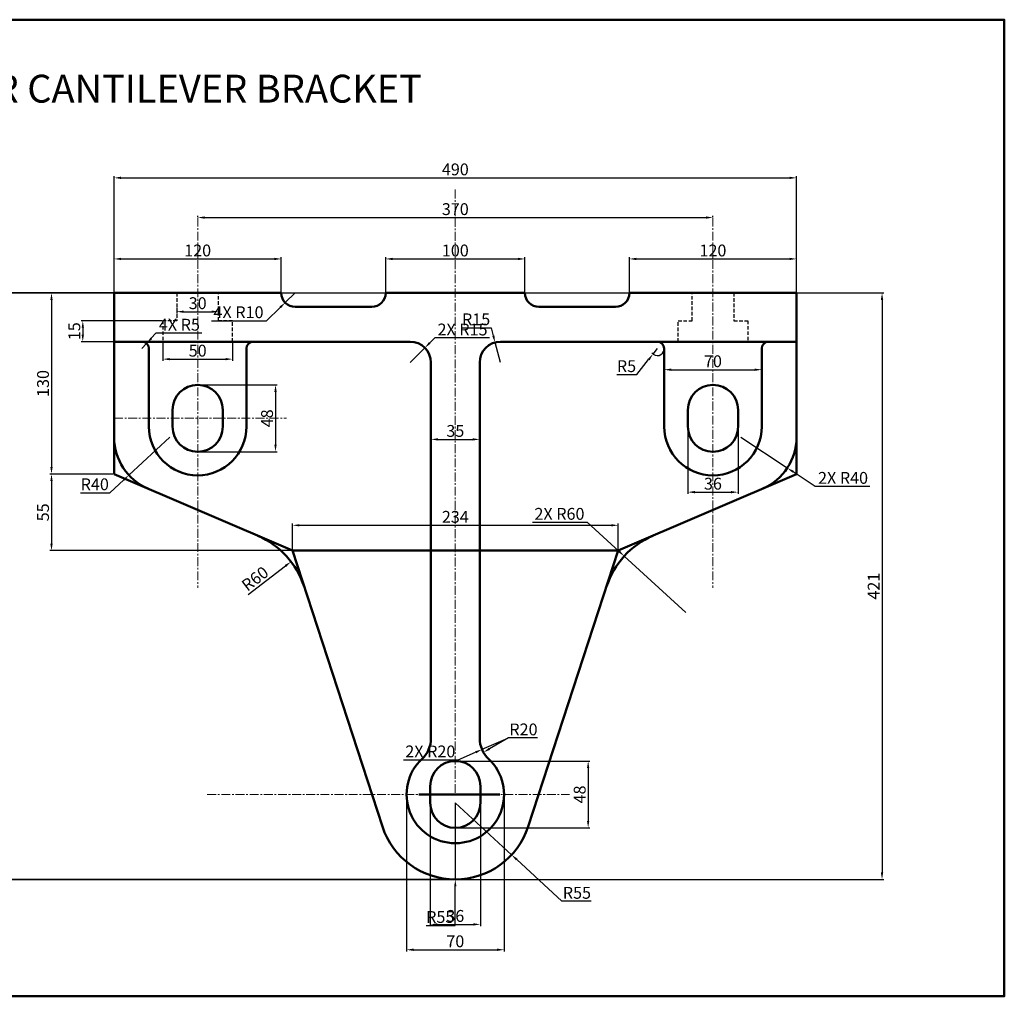
# Model space of a CAD drawing. Units: millimetres. Extents: x -624 to 605, y 670 to 1371.
# Tile 2 of 2: x -102 to 605, y 670 to 1371. Entities that reach past the tile are written whole.
import ezdxf

# ---------------------------------------------------------------- set-up
doc = ezdxf.new("R2010")
doc.units = ezdxf.units.MM
doc.header["$LTSCALE"] = 0.2
doc.linetypes.add('CENTER', pattern=[50.8, 31.75, -6.35, 6.35, -6.35])
doc.linetypes.add('DASHED', pattern=[19.05, 12.7, -6.35])
for name, color, linetype, lineweight in [('M-CNTR', 1, 'CENTER', 18), ('M-DIMS', 2, 'Continuous', 25), ('M-HIDN', 4, 'DASHED', 25), ('M-OUTL', 7, 'Continuous', 50), ('M-TEXT', 7, 'Continuous', 25)]:
    doc.layers.add(name, color=color, linetype=linetype, lineweight=lineweight)
doc.styles.get("Standard").update_dxf_attribs({"font": 'arial.ttf'})
doc.dimstyles.new('ISO-25', dxfattribs={"dimtxt": 8.5, "dimasz": 5, "dimexe": 1.25, "dimexo": 0.625, "dimtad": 1, "dimtoh": 1, "dimtxsty": 'Standard', "dimcen": 2.5, "dimadec": 0, "dimazin": 0, "dimtfac": 1, "dimtmove": 0, "dimatfit": 3, "dimfxl": 1, "dimarcsym": 0})

# ---------------------------------------------------------------- blocks, each defined once
blk = doc.blocks.new('*D22')
at = {"layer": 'Defpoints', "color": 0, "ltscale": 0.2, "transparency": 16777216}
for p in [(85.32, 1198.97), (-34.68, 1174.58), (85.32, 1174.58)]:
    blk.add_point(p, dxfattribs=at)
at = {"layer": 'M-DIMS', "color": 0, "lineweight": -2, "ltscale": 0.2, "transparency": 16777216}
for p, q in [((-34.68, 1175.21), (-34.68, 1200.22)), ((-29.68, 1198.97), (80.32, 1198.97)), ((85.32, 1175.21), (85.32, 1200.22))]:
    blk.add_line(p, q, dxfattribs=at)
at = {"layer": 'M-DIMS', "color": 0, "ltscale": 0.2, "transparency": 16777216}
for points in [[(-29.68, 1199.8), (-29.68, 1198.14), (-34.68, 1198.97)], [(80.32, 1199.8), (80.32, 1198.14), (85.32, 1198.97)]]:
    blk.add_solid(points, dxfattribs=at)
at = {"layer": 'M-DIMS', "color": 0, "ltscale": 0.2, "transparency": 16777216, "insert": (25.32, 1203.94), "char_height": 8.5, "attachment_point": 5}
blk.add_mtext('120', dxfattribs=at)
blk = doc.blocks.new('*D23')
at = {"layer": 'Defpoints', "color": 0, "ltscale": 0.2, "transparency": 16777216}
for p in [(260.32, 1198.97), (160.32, 1174.58), (260.32, 1174.58)]:
    blk.add_point(p, dxfattribs=at)
at = {"layer": 'M-DIMS', "color": 0, "lineweight": -2, "ltscale": 0.2, "transparency": 16777216}
for p, q in [((160.32, 1175.21), (160.32, 1200.22)), ((165.32, 1198.97), (255.32, 1198.97)), ((260.32, 1175.21), (260.32, 1200.22))]:
    blk.add_line(p, q, dxfattribs=at)
at = {"layer": 'M-DIMS', "color": 0, "ltscale": 0.2, "transparency": 16777216}
for points in [[(165.32, 1199.8), (165.32, 1198.14), (160.32, 1198.97)], [(255.32, 1199.8), (255.32, 1198.14), (260.32, 1198.97)]]:
    blk.add_solid(points, dxfattribs=at)
at = {"layer": 'M-DIMS', "color": 0, "ltscale": 0.2, "transparency": 16777216, "insert": (210.32, 1203.94), "char_height": 8.5, "attachment_point": 5}
blk.add_mtext('100', dxfattribs=at)
blk = doc.blocks.new('*D24')
at = {"layer": 'Defpoints', "color": 0, "ltscale": 0.2, "transparency": 16777216}
for p in [(455.32, 1198.97), (335.32, 1174.58), (455.32, 1174.58)]:
    blk.add_point(p, dxfattribs=at)
at = {"layer": 'M-DIMS', "color": 0, "lineweight": -2, "ltscale": 0.2, "transparency": 16777216}
for p, q in [((335.32, 1175.21), (335.32, 1200.22)), ((340.32, 1198.97), (450.32, 1198.97)), ((455.32, 1175.21), (455.32, 1200.22))]:
    blk.add_line(p, q, dxfattribs=at)
at = {"layer": 'M-DIMS', "color": 0, "ltscale": 0.2, "transparency": 16777216}
for points in [[(340.32, 1199.8), (340.32, 1198.14), (335.32, 1198.97)], [(450.32, 1199.8), (450.32, 1198.14), (455.32, 1198.97)]]:
    blk.add_solid(points, dxfattribs=at)
at = {"layer": 'M-DIMS', "color": 0, "ltscale": 0.2, "transparency": 16777216, "insert": (395.32, 1203.94), "char_height": 8.5, "attachment_point": 5}
blk.add_mtext('120', dxfattribs=at)
blk = doc.blocks.new('*D25')
at = {"layer": 'Defpoints', "color": 0, "ltscale": 0.2, "transparency": 16777216}
for p in [(25.32, 1228.67), (395.32, 1228.67), (395.32, 1228.67)]:
    blk.add_point(p, dxfattribs=at)
at = {"layer": 'M-DIMS', "color": 0, "lineweight": -2, "ltscale": 0.2, "transparency": 16777216}
for p, q in [((25.32, 1229.29), (25.32, 1229.92)), ((30.32, 1228.67), (390.32, 1228.67)), ((395.32, 1229.29), (395.32, 1229.92))]:
    blk.add_line(p, q, dxfattribs=at)
at = {"layer": 'M-DIMS', "color": 0, "ltscale": 0.2, "transparency": 16777216}
for points in [[(30.32, 1229.5), (30.32, 1227.83), (25.32, 1228.67)], [(390.32, 1229.5), (390.32, 1227.83), (395.32, 1228.67)]]:
    blk.add_solid(points, dxfattribs=at)
at = {"layer": 'M-DIMS', "color": 0, "ltscale": 0.2, "transparency": 16777216, "insert": (210.32, 1233.63), "char_height": 8.5, "attachment_point": 5}
blk.add_mtext('370', dxfattribs=at)
blk = doc.blocks.new('*D26')
at = {"layer": 'Defpoints', "color": 0, "ltscale": 0.2, "transparency": 16777216}
for p in [(0.32, 1154.58), (-57.18, 1139.58), (0.32, 1139.58)]:
    blk.add_point(p, dxfattribs=at)
at = {"layer": 'M-DIMS', "color": 0, "lineweight": -2, "ltscale": 0.2, "transparency": 16777216}
for p, q in [((-0.3, 1154.58), (-58.43, 1154.58)), ((-57.18, 1149.58), (-57.18, 1144.58)), ((-0.3, 1139.58), (-58.43, 1139.58))]:
    blk.add_line(p, q, dxfattribs=at)
at = {"layer": 'M-DIMS', "color": 0, "ltscale": 0.2, "transparency": 16777216}
for points in [[(-58.01, 1149.58), (-56.35, 1149.58), (-57.18, 1154.58)], [(-58.01, 1144.58), (-56.35, 1144.58), (-57.18, 1139.58)]]:
    blk.add_solid(points, dxfattribs=at)
at = {"layer": 'M-DIMS', "color": 0, "ltscale": 0.2, "transparency": 16777216, "insert": (-62.15, 1147.08), "char_height": 8.5, "attachment_point": 5, "rotation": 90}
blk.add_mtext('15', dxfattribs=at)
blk = doc.blocks.new('*D27')
at = {"layer": 'Defpoints', "color": 0, "ltscale": 0.2, "transparency": 16777216}
for p in [(10.32, 1164.58), (40.32, 1164.58), (40.32, 1161.12)]:
    blk.add_point(p, dxfattribs=at)
at = {"layer": 'M-DIMS', "color": 0, "lineweight": -2, "ltscale": 0.2, "transparency": 16777216}
for p, q in [((10.32, 1163.96), (10.32, 1159.87)), ((15.32, 1161.12), (35.32, 1161.12)), ((40.32, 1163.96), (40.32, 1159.87))]:
    blk.add_line(p, q, dxfattribs=at)
at = {"layer": 'M-DIMS', "color": 0, "ltscale": 0.2, "transparency": 16777216}
for points in [[(15.32, 1161.95), (15.32, 1160.29), (10.32, 1161.12)], [(35.32, 1161.95), (35.32, 1160.29), (40.32, 1161.12)]]:
    blk.add_solid(points, dxfattribs=at)
at = {"layer": 'M-DIMS', "color": 0, "ltscale": 0.2, "transparency": 16777216, "insert": (25.32, 1166.09), "char_height": 8.5, "attachment_point": 5}
blk.add_mtext('30', dxfattribs=at)
blk = doc.blocks.new('*D28')
at = {"layer": 'Defpoints', "color": 0, "ltscale": 0.2, "transparency": 16777216}
for p in [(0.32, 1139.58), (50.32, 1139.58), (50.32, 1127.06)]:
    blk.add_point(p, dxfattribs=at)
at = {"layer": 'M-DIMS', "color": 0, "lineweight": -2, "ltscale": 0.2, "transparency": 16777216}
for p, q in [((0.32, 1138.96), (0.32, 1125.81)), ((50.32, 1138.96), (50.32, 1125.81)), ((5.32, 1127.06), (45.32, 1127.06))]:
    blk.add_line(p, q, dxfattribs=at)
at = {"layer": 'M-DIMS', "color": 0, "ltscale": 0.2, "transparency": 16777216}
for points in [[(5.32, 1127.89), (5.32, 1126.23), (0.32, 1127.06)], [(45.32, 1127.89), (45.32, 1126.23), (50.32, 1127.06)]]:
    blk.add_solid(points, dxfattribs=at)
at = {"layer": 'M-DIMS', "color": 0, "ltscale": 0.2, "transparency": 16777216, "insert": (25.32, 1132.03), "char_height": 8.5, "attachment_point": 5}
blk.add_mtext('50', dxfattribs=at)
blk = doc.blocks.new('*D29')
at = {"layer": 'Defpoints', "color": 0, "ltscale": 0.2, "transparency": 16777216}
for p in [(-34.68, 1174.58), (-79.66, 1044.58), (-34.68, 1044.58)]:
    blk.add_point(p, dxfattribs=at)
at = {"layer": 'M-DIMS', "color": 0, "lineweight": -2, "ltscale": 0.2, "transparency": 16777216}
for p, q in [((-35.3, 1174.58), (-80.91, 1174.58)), ((-79.66, 1169.58), (-79.66, 1049.58)), ((-35.3, 1044.58), (-80.91, 1044.58))]:
    blk.add_line(p, q, dxfattribs=at)
at = {"layer": 'M-DIMS', "color": 0, "ltscale": 0.2, "transparency": 16777216}
for points in [[(-80.49, 1169.58), (-78.83, 1169.58), (-79.66, 1174.58)], [(-80.49, 1049.58), (-78.83, 1049.58), (-79.66, 1044.58)]]:
    blk.add_solid(points, dxfattribs=at)
at = {"layer": 'M-DIMS', "color": 0, "ltscale": 0.2, "transparency": 16777216, "insert": (-84.63, 1109.58), "char_height": 8.5, "attachment_point": 5, "rotation": 90}
blk.add_mtext('130', dxfattribs=at)
blk = doc.blocks.new('*D30')
at = {"layer": 'Defpoints', "color": 0, "ltscale": 0.2, "transparency": 16777216}
for p in [(-34.68, 1044.58), (-79.66, 989.58), (93.32, 989.58)]:
    blk.add_point(p, dxfattribs=at)
at = {"layer": 'M-DIMS', "color": 0, "lineweight": -2, "ltscale": 0.2, "transparency": 16777216}
for p, q in [((-35.3, 1044.58), (-80.91, 1044.58)), ((-79.66, 1039.58), (-79.66, 994.58)), ((92.7, 989.58), (-80.91, 989.58))]:
    blk.add_line(p, q, dxfattribs=at)
at = {"layer": 'M-DIMS', "color": 0, "ltscale": 0.2, "transparency": 16777216}
for points in [[(-80.49, 1039.58), (-78.83, 1039.58), (-79.66, 1044.58)], [(-80.49, 994.58), (-78.83, 994.58), (-79.66, 989.58)]]:
    blk.add_solid(points, dxfattribs=at)
at = {"layer": 'M-DIMS', "color": 0, "ltscale": 0.2, "transparency": 16777216, "insert": (-84.61, 1017.08), "char_height": 8.5, "attachment_point": 5, "rotation": 90}
blk.add_mtext('55', dxfattribs=at)
blk = doc.blocks.new('*D31')
at = {"layer": 'Defpoints', "color": 0, "ltscale": 0.2, "transparency": 16777216}
for p in [(327.32, 1007.77), (93.32, 989.58), (327.32, 989.58)]:
    blk.add_point(p, dxfattribs=at)
at = {"layer": 'M-DIMS', "color": 0, "lineweight": -2, "ltscale": 0.2, "transparency": 16777216}
for p, q in [((93.32, 990.21), (93.32, 1009.02)), ((98.32, 1007.77), (322.32, 1007.77)), ((327.32, 990.21), (327.32, 1009.02))]:
    blk.add_line(p, q, dxfattribs=at)
at = {"layer": 'M-DIMS', "color": 0, "ltscale": 0.2, "transparency": 16777216}
for points in [[(98.32, 1008.61), (98.32, 1006.94), (93.32, 1007.77)], [(322.32, 1008.61), (322.32, 1006.94), (327.32, 1007.77)]]:
    blk.add_solid(points, dxfattribs=at)
at = {"layer": 'M-DIMS', "color": 0, "ltscale": 0.2, "transparency": 16777216, "insert": (210.32, 1012.74), "char_height": 8.5, "attachment_point": 5}
blk.add_mtext('234', dxfattribs=at)
blk = doc.blocks.new('*D32')
at = {"layer": 'Defpoints', "color": 0, "ltscale": 0.2, "transparency": 16777216}
for p in [(192.82, 1076.92), (227.82, 1076.92), (227.82, 1069.44)]:
    blk.add_point(p, dxfattribs=at)
at = {"layer": 'M-DIMS', "color": 0, "lineweight": -2, "ltscale": 0.2, "transparency": 16777216}
for p, q in [((192.82, 1076.29), (192.82, 1068.19)), ((227.82, 1076.29), (227.82, 1068.19)), ((197.82, 1069.44), (222.82, 1069.44))]:
    blk.add_line(p, q, dxfattribs=at)
at = {"layer": 'M-DIMS', "color": 0, "ltscale": 0.2, "transparency": 16777216}
for points in [[(197.82, 1070.28), (197.82, 1068.61), (192.82, 1069.44)], [(222.82, 1070.28), (222.82, 1068.61), (227.82, 1069.44)]]:
    blk.add_solid(points, dxfattribs=at)
at = {"layer": 'M-DIMS', "color": 0, "ltscale": 0.2, "transparency": 16777216, "insert": (210.32, 1074.41), "char_height": 8.5, "attachment_point": 5}
blk.add_mtext('35', dxfattribs=at)
blk = doc.blocks.new('*D33')
at = {"layer": 'Defpoints', "color": 0, "ltscale": 0.2, "transparency": 16777216}
for p in [(192.32, 814.58), (228.32, 814.58), (228.32, 721.31)]:
    blk.add_point(p, dxfattribs=at)
at = {"layer": 'M-DIMS', "color": 0, "lineweight": -2, "ltscale": 0.2, "transparency": 16777216}
for p, q in [((192.32, 813.96), (192.32, 720.06)), ((228.32, 813.96), (228.32, 720.06)), ((197.32, 721.31), (223.32, 721.31))]:
    blk.add_line(p, q, dxfattribs=at)
at = {"layer": 'M-DIMS', "color": 0, "ltscale": 0.2, "transparency": 16777216}
for points in [[(197.32, 722.15), (197.32, 720.48), (192.32, 721.31)], [(223.32, 722.15), (223.32, 720.48), (228.32, 721.31)]]:
    blk.add_solid(points, dxfattribs=at)
at = {"layer": 'M-DIMS', "color": 0, "ltscale": 0.2, "transparency": 16777216, "insert": (210.32, 726.28), "char_height": 8.5, "attachment_point": 5}
blk.add_mtext('36', dxfattribs=at)
blk = doc.blocks.new('*D34')
at = {"layer": 'Defpoints', "color": 0, "ltscale": 0.2, "transparency": 16777216}
for p in [(175.32, 814.58), (245.32, 814.58), (245.32, 703.11)]:
    blk.add_point(p, dxfattribs=at)
at = {"layer": 'M-DIMS', "color": 0, "lineweight": -2, "ltscale": 0.2, "transparency": 16777216}
for p, q in [((175.32, 813.96), (175.32, 701.86)), ((245.32, 813.96), (245.32, 701.86)), ((180.32, 703.11), (240.32, 703.11))]:
    blk.add_line(p, q, dxfattribs=at)
at = {"layer": 'M-DIMS', "color": 0, "ltscale": 0.2, "transparency": 16777216}
for points in [[(180.32, 703.94), (180.32, 702.27), (175.32, 703.11)], [(240.32, 703.94), (240.32, 702.27), (245.32, 703.11)]]:
    blk.add_solid(points, dxfattribs=at)
at = {"layer": 'M-DIMS', "color": 0, "ltscale": 0.2, "transparency": 16777216, "insert": (210.32, 708.07), "char_height": 8.5, "attachment_point": 5}
blk.add_mtext('70', dxfattribs=at)
blk = doc.blocks.new('*D35')
at = {"layer": 'Defpoints', "color": 0, "ltscale": 0.2, "transparency": 16777216}
for p in [(210.32, 838.58), (210.32, 790.58), (305.7, 790.58)]:
    blk.add_point(p, dxfattribs=at)
at = {"layer": 'M-DIMS', "color": 0, "lineweight": -2, "ltscale": 0.2, "transparency": 16777216}
for p, q in [((210.95, 838.58), (306.95, 838.58)), ((305.7, 833.58), (305.7, 795.58)), ((210.95, 790.58), (306.95, 790.58))]:
    blk.add_line(p, q, dxfattribs=at)
at = {"layer": 'M-DIMS', "color": 0, "ltscale": 0.2, "transparency": 16777216}
for points in [[(304.87, 833.58), (306.53, 833.58), (305.7, 838.58)], [(304.87, 795.58), (306.53, 795.58), (305.7, 790.58)]]:
    blk.add_solid(points, dxfattribs=at)
at = {"layer": 'M-DIMS', "color": 0, "ltscale": 0.2, "transparency": 16777216, "insert": (300.74, 814.58), "char_height": 8.5, "attachment_point": 5, "rotation": 90}
blk.add_mtext('48', dxfattribs=at)
blk = doc.blocks.new('*D36')
at = {"layer": 'Defpoints', "color": 0, "ltscale": 0.2, "transparency": 16777216}
for p in [(247.82, 854.81), (230.5, 844.81)]:
    blk.add_point(p, dxfattribs=at)
at = {"layer": 'M-DIMS', "color": 0, "lineweight": -2, "ltscale": 0.2, "transparency": 16777216}
for p, q in [((248.48, 855.2), (234.83, 847.31)), ((269.39, 855.2), (248.48, 855.2))]:
    blk.add_line(p, q, dxfattribs=at)
at = {"layer": 'M-DIMS', "color": 0, "ltscale": 0.2, "transparency": 16777216}
blk.add_solid([(234.41, 848.04), (235.25, 846.59), (230.5, 844.81)], dxfattribs=at)
at = {"layer": 'M-DIMS', "color": 0, "ltscale": 0.2, "transparency": 16777216, "insert": (259.25, 860.16), "char_height": 8.5, "attachment_point": 5}
blk.add_mtext('R20', dxfattribs=at)
blk = doc.blocks.new('*D37')
at = {"layer": 'Defpoints', "color": 0, "ltscale": 0.2, "transparency": 16777216}
for p in [(210.32, 808.58), (250.72, 771.26)]:
    blk.add_point(p, dxfattribs=at)
at = {"layer": 'M-DIMS', "color": 0, "lineweight": -2, "ltscale": 0.2, "transparency": 16777216}
for p, q in [((210.32, 808.58), (250.72, 771.26)), ((286.82, 737.92), (254.4, 767.87)), ((307.82, 737.92), (286.82, 737.92))]:
    blk.add_line(p, q, dxfattribs=at)
at = {"layer": 'M-DIMS', "color": 0, "ltscale": 0.2, "transparency": 16777216}
blk.add_solid([(254.96, 768.48), (253.83, 767.26), (250.72, 771.26)], dxfattribs=at)
at = {"layer": 'M-DIMS', "color": 0, "ltscale": 0.2, "transparency": 16777216, "insert": (297.63, 742.87), "char_height": 8.5, "attachment_point": 5}
blk.add_mtext('R55', dxfattribs=at)
blk = doc.blocks.new('*D38')
at = {"layer": 'Defpoints', "color": 0, "ltscale": 0.2, "transparency": 16777216}
for p in [(92.35, 981.64), (44.71, 945.16)]:
    blk.add_point(p, dxfattribs=at)
at = {"layer": 'M-DIMS', "color": 0, "lineweight": -2, "ltscale": 0.2, "transparency": 16777216}
blk.add_line((61.62, 958.11), (88.38, 978.6), dxfattribs=at)
at = {"layer": 'M-DIMS', "color": 0, "ltscale": 0.2, "transparency": 16777216}
blk.add_solid([(87.87, 979.26), (88.89, 977.94), (92.35, 981.64)], dxfattribs=at)
at = {"layer": 'M-DIMS', "color": 0, "ltscale": 0.2, "transparency": 16777216, "insert": (67.15, 968.6), "char_height": 8.5, "attachment_point": 5, "rotation": 37.44326}
blk.add_mtext('R60', dxfattribs=at)
blk = doc.blocks.new('*D39')
at = {"layer": 'Defpoints', "color": 0, "ltscale": 0.2, "transparency": 16777216}
for p in [(5.32, 1070.93), (-24.08, 1043.81)]:
    blk.add_point(p, dxfattribs=at)
at = {"layer": 'M-DIMS', "color": 0, "lineweight": -2, "ltscale": 0.2, "transparency": 16777216}
for p, q in [((5.32, 1070.93), (-24.08, 1043.81)), ((-37.81, 1031.14), (-27.76, 1040.42)), ((-58.72, 1031.14), (-37.81, 1031.14))]:
    blk.add_line(p, q, dxfattribs=at)
at = {"layer": 'M-DIMS', "color": 0, "ltscale": 0.2, "transparency": 16777216}
blk.add_solid([(-28.32, 1041.03), (-27.19, 1039.81), (-24.08, 1043.81)], dxfattribs=at)
at = {"layer": 'M-DIMS', "color": 0, "ltscale": 0.2, "transparency": 16777216, "insert": (-48.58, 1036.11), "char_height": 8.5, "attachment_point": 5}
blk.add_mtext('R40', dxfattribs=at)
blk = doc.blocks.new('*D40')
at = {"layer": 'Defpoints', "color": 0, "ltscale": 0.2, "transparency": 16777216}
for p in [(25.32, 1108.58), (25.32, 1060.58), (81.21, 1060.58)]:
    blk.add_point(p, dxfattribs=at)
at = {"layer": 'M-DIMS', "color": 0, "lineweight": -2, "ltscale": 0.2, "transparency": 16777216}
for p, q in [((25.95, 1108.58), (82.46, 1108.58)), ((81.21, 1103.58), (81.21, 1065.58)), ((25.95, 1060.58), (82.46, 1060.58))]:
    blk.add_line(p, q, dxfattribs=at)
at = {"layer": 'M-DIMS', "color": 0, "ltscale": 0.2, "transparency": 16777216}
for points in [[(80.37, 1103.58), (82.04, 1103.58), (81.21, 1108.58)], [(80.37, 1065.58), (82.04, 1065.58), (81.21, 1060.58)]]:
    blk.add_solid(points, dxfattribs=at)
at = {"layer": 'M-DIMS', "color": 0, "ltscale": 0.2, "transparency": 16777216, "insert": (76.24, 1084.58), "char_height": 8.5, "attachment_point": 5, "rotation": 90}
blk.add_mtext('48', dxfattribs=at)
blk = doc.blocks.new('*D41')
at = {"layer": 'Defpoints', "color": 0, "ltscale": 0.2, "transparency": 16777216}
for p in [(455.32, 1257.18), (-34.68, 1174.58), (455.32, 1174.58)]:
    blk.add_point(p, dxfattribs=at)
at = {"layer": 'M-DIMS', "color": 0, "lineweight": -2, "ltscale": 0.2, "transparency": 16777216}
for p, q in [((-34.68, 1175.21), (-34.68, 1258.43)), ((-29.68, 1257.18), (450.32, 1257.18)), ((455.32, 1175.21), (455.32, 1258.43))]:
    blk.add_line(p, q, dxfattribs=at)
at = {"layer": 'M-DIMS', "color": 0, "ltscale": 0.2, "transparency": 16777216}
for points in [[(-29.68, 1258.02), (-29.68, 1256.35), (-34.68, 1257.18)], [(450.32, 1258.02), (450.32, 1256.35), (455.32, 1257.18)]]:
    blk.add_solid(points, dxfattribs=at)
at = {"layer": 'M-DIMS', "color": 0, "ltscale": 0.2, "transparency": 16777216, "insert": (210.32, 1262.15), "char_height": 8.5, "attachment_point": 5}
blk.add_mtext('490', dxfattribs=at)
blk = doc.blocks.new('*D42')
at = {"layer": 'Defpoints', "color": 0, "ltscale": 0.2, "transparency": 16777216}
for p in [(360.32, 1118.8), (430.32, 1119.47), (430.32, 1118.8)]:
    blk.add_point(p, dxfattribs=at)
at = {"layer": 'M-DIMS', "color": 0, "lineweight": -2, "ltscale": 0.2, "transparency": 16777216}
for p, q in [((360.32, 1119.42), (360.32, 1120.72)), ((365.32, 1119.47), (425.32, 1119.47)), ((430.32, 1119.42), (430.32, 1120.72))]:
    blk.add_line(p, q, dxfattribs=at)
at = {"layer": 'M-DIMS', "color": 0, "ltscale": 0.2, "transparency": 16777216}
for points in [[(365.32, 1120.3), (365.32, 1118.64), (360.32, 1119.47)], [(425.32, 1120.3), (425.32, 1118.64), (430.32, 1119.47)]]:
    blk.add_solid(points, dxfattribs=at)
at = {"layer": 'M-DIMS', "color": 0, "ltscale": 0.2, "transparency": 16777216, "insert": (395.32, 1124.43), "char_height": 8.5, "attachment_point": 5}
blk.add_mtext('70', dxfattribs=at)
blk = doc.blocks.new('*D43')
at = {"layer": 'Defpoints', "color": 0, "ltscale": 0.2, "transparency": 16777216}
for p in [(377.32, 1084.58), (413.32, 1084.58), (413.32, 1031.58)]:
    blk.add_point(p, dxfattribs=at)
at = {"layer": 'M-DIMS', "color": 0, "lineweight": -2, "ltscale": 0.2, "transparency": 16777216}
for p, q in [((377.32, 1083.96), (377.32, 1030.33)), ((413.32, 1083.96), (413.32, 1030.33)), ((382.32, 1031.58), (408.32, 1031.58))]:
    blk.add_line(p, q, dxfattribs=at)
at = {"layer": 'M-DIMS', "color": 0, "ltscale": 0.2, "transparency": 16777216}
for points in [[(382.32, 1032.41), (382.32, 1030.75), (377.32, 1031.58)], [(408.32, 1032.41), (408.32, 1030.75), (413.32, 1031.58)]]:
    blk.add_solid(points, dxfattribs=at)
at = {"layer": 'M-DIMS', "color": 0, "ltscale": 0.2, "transparency": 16777216, "insert": (395.32, 1036.55), "char_height": 8.5, "attachment_point": 5}
blk.add_mtext('36', dxfattribs=at)
blk = doc.blocks.new('*D44')
at = {"layer": 'Defpoints', "color": 0, "ltscale": 0.2, "transparency": 16777216}
for p in [(355.32, 1134.58), (352.24, 1130.64)]:
    blk.add_point(p, dxfattribs=at)
at = {"layer": 'M-DIMS', "color": 0, "lineweight": -2, "ltscale": 0.2, "transparency": 16777216}
for p, q in [((355.32, 1134.58), (352.24, 1130.64)), ((340.74, 1115.97), (349.15, 1126.71)), ((326.34, 1115.97), (340.74, 1115.97))]:
    blk.add_line(p, q, dxfattribs=at)
blk.add_arc((355.32, 1134.58), 5, 217.60221, 352.83803, dxfattribs=at)
at = {"layer": 'M-DIMS', "color": 0, "ltscale": 0.2, "transparency": 16777216}
blk.add_solid([(348.5, 1127.22), (349.81, 1126.19), (352.24, 1130.64)], dxfattribs=at)
at = {"layer": 'M-DIMS', "color": 0, "ltscale": 0.2, "transparency": 16777216, "insert": (333.23, 1120.91), "char_height": 8.5, "attachment_point": 5}
blk.add_mtext('R5', dxfattribs=at)
blk = doc.blocks.new('*D45')
at = {"layer": 'Defpoints', "color": 0, "ltscale": 0.2, "transparency": 16777216}
for p in [(238.89, 1139.06), (242.82, 1124.58)]:
    blk.add_point(p, dxfattribs=at)
at = {"layer": 'M-DIMS', "color": 0, "lineweight": -2, "ltscale": 0.2, "transparency": 16777216}
for p, q in [((215.05, 1149.54), (236.05, 1149.54)), ((236.05, 1149.54), (237.58, 1143.88)), ((242.82, 1124.58), (238.89, 1139.06))]:
    blk.add_line(p, q, dxfattribs=at)
at = {"layer": 'M-DIMS', "color": 0, "ltscale": 0.2, "transparency": 16777216}
blk.add_solid([(238.39, 1144.1), (236.78, 1143.66), (238.89, 1139.06)], dxfattribs=at)
at = {"layer": 'M-DIMS', "color": 0, "ltscale": 0.2, "transparency": 16777216, "insert": (225.24, 1154.51), "char_height": 8.5, "attachment_point": 5}
blk.add_mtext('R15', dxfattribs=at)
blk = doc.blocks.new('*D47')
at = {"layer": 'Defpoints', "color": 0, "ltscale": 0.2, "transparency": 16777216}
for p in [(-548.12, 1174.58), (-188.12, 753.58), (516.74, 753.58)]:
    blk.add_point(p, dxfattribs=at)
at = {"layer": 'M-DIMS', "color": 0, "lineweight": -2, "ltscale": 0.2, "transparency": 16777216}
for p, q in [((-547.5, 1174.58), (517.99, 1174.58)), ((516.74, 1169.58), (516.74, 758.58)), ((-187.5, 753.58), (517.99, 753.58))]:
    blk.add_line(p, q, dxfattribs=at)
at = {"layer": 'M-DIMS', "color": 0, "ltscale": 0.2, "transparency": 16777216}
for points in [[(515.9, 1169.58), (517.57, 1169.58), (516.74, 1174.58)], [(515.9, 758.58), (517.57, 758.58), (516.74, 753.58)]]:
    blk.add_solid(points, dxfattribs=at)
at = {"layer": 'M-DIMS', "color": 0, "ltscale": 0.2, "transparency": 16777216, "insert": (511.84, 964.08), "char_height": 8.5, "attachment_point": 5, "rotation": 90}
blk.add_mtext('421', dxfattribs=at)
blk = doc.blocks.new('*D48')
at = {"layer": 'Defpoints', "color": 0, "ltscale": 0.2, "transparency": 16777216}
for p in [(-34.68, 1174.58), (-609.54, 753.58), (210.32, 753.58)]:
    blk.add_point(p, dxfattribs=at)
at = {"layer": 'M-DIMS', "color": 0, "lineweight": -2, "ltscale": 0.2, "transparency": 16777216}
for p, q in [((-35.3, 1174.58), (-610.79, 1174.58)), ((-609.54, 1169.58), (-609.54, 758.58)), ((209.7, 753.58), (-610.79, 753.58))]:
    blk.add_line(p, q, dxfattribs=at)
at = {"layer": 'M-DIMS', "color": 0, "ltscale": 0.2, "transparency": 16777216}
for points in [[(-610.37, 1169.58), (-608.71, 1169.58), (-609.54, 1174.58)], [(-610.37, 758.58), (-608.71, 758.58), (-609.54, 753.58)]]:
    blk.add_solid(points, dxfattribs=at)
at = {"layer": 'M-DIMS', "color": 0, "ltscale": 0.2, "transparency": 16777216, "insert": (-614.43, 964.08), "char_height": 8.5, "attachment_point": 5, "rotation": 90}
blk.add_mtext('421', dxfattribs=at)
blk = doc.blocks.new('*D54')
at = {"layer": 'Defpoints', "color": 0, "ltscale": 0.2, "transparency": 16777216}
for p in [(188.43, 1135.19), (177.82, 1124.58)]:
    blk.add_point(p, dxfattribs=at)
at = {"layer": 'M-DIMS', "color": 0, "lineweight": -2, "ltscale": 0.2, "transparency": 16777216}
for p, q in [((195.5, 1142.26), (191.96, 1138.72)), ((234.91, 1142.26), (195.5, 1142.26)), ((177.82, 1124.58), (188.43, 1135.19))]:
    blk.add_line(p, q, dxfattribs=at)
at = {"layer": 'M-DIMS', "color": 0, "ltscale": 0.2, "transparency": 16777216}
blk.add_solid([(191.37, 1139.31), (192.55, 1138.13), (188.43, 1135.19)], dxfattribs=at)
at = {"layer": 'M-DIMS', "color": 0, "ltscale": 0.2, "transparency": 16777216, "insert": (215.51, 1147.22), "char_height": 8.5, "attachment_point": 5}
blk.add_mtext('2X R15', dxfattribs=at)
blk = doc.blocks.new('*D55')
at = {"layer": 'Defpoints', "color": 0, "ltscale": 0.2, "transparency": 16777216}
for p in [(-14.68, 1134.58), (-11.33, 1138.29)]:
    blk.add_point(p, dxfattribs=at)
at = {"layer": 'M-DIMS', "color": 0, "lineweight": -2, "ltscale": 0.2, "transparency": 16777216}
for p, q in [((-4.62, 1145.71), (-7.98, 1142)), ((28.38, 1145.71), (-4.62, 1145.71)), ((-14.68, 1134.58), (-11.33, 1138.29))]:
    blk.add_line(p, q, dxfattribs=at)
at = {"layer": 'M-DIMS', "color": 0, "ltscale": 0.2, "transparency": 16777216}
blk.add_solid([(-8.59, 1142.56), (-7.36, 1141.44), (-11.33, 1138.29)], dxfattribs=at)
at = {"layer": 'M-DIMS', "color": 0, "ltscale": 0.2, "transparency": 16777216, "insert": (12.19, 1150.66), "char_height": 8.5, "attachment_point": 5}
blk.add_mtext('4X R5', dxfattribs=at)
blk = doc.blocks.new('*D56')
at = {"layer": 'Defpoints', "color": 0, "ltscale": 0.2, "transparency": 16777216}
for p in [(95.32, 1174.58), (88.13, 1167.63)]:
    blk.add_point(p, dxfattribs=at)
at = {"layer": 'M-DIMS', "color": 0, "lineweight": -2, "ltscale": 0.2, "transparency": 16777216}
for p, q in [((95.32, 1174.58), (88.13, 1167.63)), ((74.71, 1154.64), (84.54, 1164.15)), ((35.19, 1154.64), (74.71, 1154.64))]:
    blk.add_line(p, q, dxfattribs=at)
at = {"layer": 'M-DIMS', "color": 0, "ltscale": 0.2, "transparency": 16777216}
blk.add_solid([(83.96, 1164.75), (85.12, 1163.55), (88.13, 1167.63)], dxfattribs=at)
at = {"layer": 'M-DIMS', "color": 0, "ltscale": 0.2, "transparency": 16777216, "insert": (54.64, 1159.61), "char_height": 8.5, "attachment_point": 5}
blk.add_mtext('4X R10', dxfattribs=at)
blk = doc.blocks.new('*D57')
at = {"layer": 'Defpoints', "color": 0, "ltscale": 0.2, "transparency": 16777216}
for p in [(415.32, 1070.93), (448.73, 1048.93)]:
    blk.add_point(p, dxfattribs=at)
at = {"layer": 'M-DIMS', "color": 0, "lineweight": -2, "ltscale": 0.2, "transparency": 16777216}
for p, q in [((415.32, 1070.93), (448.73, 1048.93)), ((468.77, 1035.73), (452.9, 1046.18)), ((508.09, 1035.73), (468.77, 1035.73))]:
    blk.add_line(p, q, dxfattribs=at)
at = {"layer": 'M-DIMS', "color": 0, "ltscale": 0.2, "transparency": 16777216}
blk.add_solid([(453.36, 1046.88), (452.45, 1045.49), (448.73, 1048.93)], dxfattribs=at)
at = {"layer": 'M-DIMS', "color": 0, "ltscale": 0.2, "transparency": 16777216, "insert": (488.74, 1040.7), "char_height": 8.5, "attachment_point": 5}
blk.add_mtext('2X R40', dxfattribs=at)
blk = doc.blocks.new('*D58')
at = {"layer": 'Defpoints', "color": 0, "ltscale": 0.2, "transparency": 16777216}
for p in [(331.64, 985.64), (375.93, 945.16)]:
    blk.add_point(p, dxfattribs=at)
at = {"layer": 'M-DIMS', "color": 0, "lineweight": -2, "ltscale": 0.2, "transparency": 16777216}
for p, q in [((265.75, 1009.93), (305.07, 1009.93)), ((305.07, 1009.93), (327.95, 989.01)), ((375.93, 945.16), (331.64, 985.64))]:
    blk.add_line(p, q, dxfattribs=at)
at = {"layer": 'M-DIMS', "color": 0, "ltscale": 0.2, "transparency": 16777216}
blk.add_solid([(328.51, 989.63), (327.39, 988.4), (331.64, 985.64)], dxfattribs=at)
at = {"layer": 'M-DIMS', "color": 0, "ltscale": 0.2, "transparency": 16777216, "insert": (285.1, 1014.89), "char_height": 8.5, "attachment_point": 5}
blk.add_mtext('2X R60', dxfattribs=at)
blk = doc.blocks.new('*D59')
at = {"layer": 'Defpoints', "color": 0, "ltscale": 0.2, "transparency": 16777216}
for p in [(210.32, 808.58), (210.32, 753.58)]:
    blk.add_point(p, dxfattribs=at)
at = {"layer": 'M-DIMS', "color": 0, "lineweight": -2, "ltscale": 0.2, "transparency": 16777216}
for p, q in [((210.32, 808.58), (210.32, 753.58)), ((210.32, 720.58), (210.32, 748.58)), ((189.32, 720.58), (210.32, 720.58))]:
    blk.add_line(p, q, dxfattribs=at)
at = {"layer": 'M-DIMS', "color": 0, "ltscale": 0.2, "transparency": 16777216}
blk.add_solid([(209.49, 748.58), (211.15, 748.58), (210.32, 753.58)], dxfattribs=at)
at = {"layer": 'M-DIMS', "color": 0, "ltscale": 0.2, "transparency": 16777216, "insert": (199.51, 725.53), "char_height": 8.5, "attachment_point": 5}
blk.add_mtext('R55', dxfattribs=at)
blk = doc.blocks.new('*D60')
at = {"layer": 'Defpoints', "color": 0, "ltscale": 0.2, "transparency": 16777216}
for p in [(247.82, 854.81), (229.48, 846.84)]:
    blk.add_point(p, dxfattribs=at)
at = {"layer": 'M-DIMS', "color": 0, "lineweight": -2, "ltscale": 0.2, "transparency": 16777216}
for p, q in [((247.82, 854.81), (229.48, 846.84)), ((212.35, 839.39), (224.89, 844.85)), ((173.03, 839.39), (212.35, 839.39))]:
    blk.add_line(p, q, dxfattribs=at)
at = {"layer": 'M-DIMS', "color": 0, "ltscale": 0.2, "transparency": 16777216}
blk.add_solid([(224.56, 845.61), (225.23, 844.08), (229.48, 846.84)], dxfattribs=at)
at = {"layer": 'M-DIMS', "color": 0, "ltscale": 0.2, "transparency": 16777216, "insert": (192.38, 844.36), "char_height": 8.5, "attachment_point": 5}
blk.add_mtext('2X R20', dxfattribs=at)

msp = doc.modelspace()

# ---------------------------------------------------------------- linework, layer by layer
at = {"layer": 'M-CNTR'}
for p, q in [((210.321, 1248.804), (210.321, 814.58)), ((25.321, 1228.667), (25.321, 962.912)), ((395.321, 1228.667), (395.321, 962.912)), ((-34.679, 1084.58), (89.084, 1084.58)), ((32.216, 814.58), (292.305, 814.58))]:
    msp.add_line(p, q, dxfattribs=at)
at = {"layer": 'M-HIDN'}
for points in [[(50.321, 1139.58), (50.321, 1154.58), (40.321, 1154.58), (40.321, 1174.58), (10.321, 1174.58), (10.321, 1154.58), (0.321, 1154.58), (0.321, 1139.58)], [(370.321, 1139.58), (370.321, 1154.58), (380.321, 1154.58), (380.321, 1174.58), (410.321, 1174.58), (410.321, 1154.58), (420.321, 1154.58), (420.321, 1139.58)]]:
    msp.add_lwpolyline(points, close=True, dxfattribs=at)
at = {"layer": 'M-OUTL'}
for p, q in [((-34.679, 1174.58), (85.321, 1174.58)), ((-34.679, 1139.58), (-34.679, 1174.58)), ((-34.679, 1174.58), (-34.679, 1139.58)), ((85.321, 1174.58), (85.321, 1174.58)), ((160.321, 1174.58), (160.321, 1174.58)), ((160.321, 1174.58), (260.321, 1174.58)), ((260.321, 1174.58), (260.321, 1174.58)), ((335.321, 1174.58), (335.321, 1174.58)), ((335.321, 1174.58), (455.321, 1174.58)), ((455.321, 1174.58), (455.321, 1139.58)), ((150.321, 1164.58), (95.321, 1164.58)), ((270.321, 1164.58), (325.321, 1164.58)), ((65.321, 1139.58), (-34.679, 1139.58)), ((-34.679, 1139.58), (-34.679, 1070.929)), ((177.821, 1139.58), (65.321, 1139.58)), ((355.321, 1139.58), (242.821, 1139.58)), ((455.321, 1139.58), (355.321, 1139.58)), ((455.321, 1139.58), (455.321, 1070.929)), ((-9.679, 1134.58), (-9.679, 1078.58)), ((60.321, 1134.58), (60.321, 1078.58)), ((360.321, 1134.58), (360.321, 1078.58)), ((430.321, 1134.58), (430.321, 1078.58)), ((192.821, 1124.58), (192.821, 854.814)), ((227.821, 1124.58), (227.821, 854.814)), ((-34.679, 1070.929), (-34.679, 1044.58)), ((455.321, 1070.929), (455.321, 1044.58)), ((-34.679, 1044.58), (93.321, 989.58)), ((455.321, 1044.58), (327.321, 989.58)), ((93.321, 989.58), (192.821, 989.58)), ((93.321, 989.58), (158.04, 791.499)), ((192.821, 989.58), (327.321, 989.58)), ((327.321, 989.58), (262.601, 791.499)), ((242.349, 814.58), (184.083, 814.58))]:
    msp.add_line(p, q, dxfattribs=at)
at = {"layer": 'M-OUTL', "ltscale": 0.2}
msp.add_lwpolyline([(-623.802, 1370.695), (604.533, 1370.695), (604.533, 669.699), (-623.802, 669.699)], close=True, dxfattribs=at)
at = {"layer": 'M-OUTL'}
for points in [[(43.321, 1090.58, 1), (7.321, 1090.58), (7.321, 1084.58), (7.321, 1078.58, 1), (43.321, 1078.58)], [(377.321, 1090.58, -1), (413.321, 1090.58), (413.321, 1084.58), (413.321, 1078.58, -1), (377.321, 1078.58)], [(228.321, 820.58, 1), (192.321, 820.58), (192.321, 814.58), (192.321, 808.58, 1), (228.321, 808.58)]]:
    msp.add_lwpolyline(points, format="xyb", close=True, dxfattribs=at)
for centre, radius, start, end in [((95.321, 1174.58), 10, 180, 270), ((150.321, 1174.58), 10, 270, 0), ((270.321, 1174.58), 10, 180, 270), ((325.321, 1174.58), 10, 270, 0), ((-14.679, 1134.58), 5, 0, 90), ((65.321, 1134.58), 5, 90, 180), ((177.821, 1124.58), 15, 0, 90), ((242.821, 1124.58), 15, 90, 180), ((355.321, 1134.58), 5, 0, 90), ((435.321, 1134.58), 5, 90, 180), ((25.321, 1078.58), 35, 180, 0), ((395.321, 1078.58), 35, 180, 0), ((5.321, 1070.929), 40, 180, 246.747408), ((415.321, 1070.929), 40, 293.252592, 0), ((44.712, 945.162), 60, 18.093926, 66.747408), ((375.929, 945.162), 60, 113.252592, 161.906074), ((172.821, 854.814), 20, 312.985886, 0), ((247.821, 854.814), 20, 180, 227.014114), ((210.321, 814.58), 35, 132.985886, 47.014114), ((210.321, 808.58), 55, 198.093926, 341.906074)]:
    msp.add_arc(centre, radius, start, end, dxfattribs=at)

# ---------------------------------------------------------------- texts
at = {"layer": 'M-TEXT', "ltscale": 0.2, "insert": (-226.692, 1331.188), "char_height": 20, "attachment_point": 1}
msp.add_mtext_dynamic_manual_height_columns('ANGULAR CANTILEVER BRACKET', width=461.44309, gutter_width=12.5, heights=[0], dxfattribs=at)

# ---------------------------------------------------------------- dimensions: what is measured, and where the dimension line sits
at = {"layer": 'M-DIMS', "ltscale": 0.2}
for base, p1, p2, picture, middle in [((455.321, 1257.185), (-34.679, 1174.58), (455.321, 1174.58), '*D41', (210.321, 1262.15)), ((395.321, 1228.667), (25.321, 1228.667), (395.321, 1228.667), '*D25', (210.321, 1233.635)), ((85.321, 1198.971), (-34.679, 1174.58), (85.321, 1174.58), '*D22', (25.321, 1203.936)), ((260.321, 1198.971), (160.321, 1174.58), (260.321, 1174.58), '*D23', (210.321, 1203.936)), ((455.321, 1198.971), (335.321, 1174.58), (455.321, 1174.58), '*D24', (395.321, 1203.936)), ((40.321, 1161.12), (10.321, 1164.58), (40.321, 1164.58), '*D27', (25.321, 1166.087)), ((50.321, 1127.061), (0.321, 1139.58), (50.321, 1139.58), '*D28', (25.321, 1132.026)), ((430.321, 1119.47), (360.321, 1118.796), (430.321, 1118.796), '*D42', (395.321, 1124.434)), ((413.321, 1031.58), (377.321, 1084.58), (413.321, 1084.58), '*D43', (395.321, 1036.548)), ((227.821, 1069.445), (192.821, 1076.916), (227.821, 1076.916), '*D32', (210.321, 1074.413)), ((327.321, 1007.774), (93.321, 989.58), (327.321, 989.58), '*D31', (210.321, 1012.741)), ((245.321, 703.107), (175.321, 814.58), (245.321, 814.58), '*D34', (210.321, 708.072)), ((228.321, 721.312), (192.321, 814.58), (228.321, 814.58), '*D33', (210.321, 726.28))]:
    dim = msp.add_linear_dim(base=base, p1=p1, p2=p2, dimstyle='ISO-25', override={"dimclrd": 0, "dimclre": 0, "dimclrt": 0}, dxfattribs=at)
    dim.commit()
    dim.dimension.update_dxf_attribs({"geometry": picture, "text_midpoint": middle})
for base, p1, p2, override, picture, middle in [((-609.541, 753.58), (-34.679, 1174.58), (210.321, 753.58), {"dimdec": 0, "dimlfac": 1, "dimrnd": 0, "dimzin": 0, "dimdsep": 46, "dimlunit": 2}, '*D48', (-614.433, 964.08)), ((516.737, 753.58), (-548.124, 1174.58), (-188.124, 753.58), {"dimdec": 0, "dimlfac": 1, "dimrnd": 0, "dimzin": 0, "dimdsep": 46, "dimlunit": 2}, '*D47', (511.845, 964.08)), ((-79.659, 1044.58), (-34.679, 1174.58), (-34.679, 1044.58), {"dimclrd": 0, "dimclre": 0, "dimclrt": 0}, '*D29', (-84.627, 1109.58)), ((-57.181, 1139.58), (0.321, 1154.58), (0.321, 1139.58), {"dimclrd": 0, "dimclre": 0, "dimclrt": 0}, '*D26', (-62.146, 1147.08)), ((81.206, 1060.58), (25.321, 1108.58), (25.321, 1060.58), {"dimclrd": 0, "dimclre": 0, "dimclrt": 0}, '*D40', (76.241, 1084.58)), ((-79.659, 989.58), (-34.679, 1044.58), (93.321, 989.58), {"dimclrd": 0, "dimclre": 0, "dimclrt": 0}, '*D30', (-84.606, 1017.08)), ((305.701, 790.58), (210.321, 838.58), (210.321, 790.58), {"dimclrd": 0, "dimclre": 0, "dimclrt": 0}, '*D35', (300.736, 814.58))]:
    dim = msp.add_linear_dim(base=base, p1=p1, p2=p2, angle=90, dimstyle='ISO-25', override=override, dxfattribs=at)
    dim.commit()
    dim.dimension.update_dxf_attribs({"geometry": picture, "text_midpoint": middle})
for center, mpoint, text, picture, middle in [((95.321, 1174.58), (88.132, 1167.628), '4X <>', '*D56', (54.636, 1159.607)), ((-14.679, 1134.58), (-11.328, 1138.291), '4X <>', '*D55', (12.189, 1150.659)), ((177.821, 1124.58), (188.427, 1135.187), '2X <>', '*D54', (215.515, 1147.223)), ((247.821, 854.814), (229.479, 846.84), '2X <>', '*D60', (192.378, 844.357))]:
    dim = msp.add_radius_dim(center=center, mpoint=mpoint, text=text, dimstyle='ISO-25', override={"dimdec": 0, "dimlfac": 1, "dimrnd": 0, "dimzin": 0, "dimdsep": 46, "dimlunit": 2}, dxfattribs=at)
    dim.commit()
    dim.dimension.update_dxf_attribs({"geometry": picture, "text_midpoint": middle})
for center, mpoint, override, picture, middle in [((242.821, 1124.58), (238.894, 1139.057), {"dimclrd": 0, "dimclre": 0, "dimclrt": 0}, '*D45', (225.237, 1149.545)), ((44.712, 945.162), (92.349, 981.641), {"dimclrd": 0, "dimclre": 0, "dimclrt": 0}, '*D38', (70.172, 964.658)), ((247.821, 854.814), (230.5, 844.814), {"dimclrd": 0, "dimclre": 0, "dimclrt": 0}, '*D36', (259.25, 855.197)), ((210.321, 808.58), (210.32, 753.58), {"dimdec": 0, "dimlfac": 1, "dimrnd": 0, "dimzin": 0, "dimdsep": 46, "dimlunit": 2}, '*D59', (199.507, 720.58)), ((210.321, 808.58), (250.723, 771.262), {"dimclrd": 0, "dimclre": 0, "dimclrt": 0}, '*D37', (297.632, 737.92))]:
    dim = msp.add_radius_dim(center=center, mpoint=mpoint, dimstyle='ISO-25', override=override, dxfattribs=at)
    dim.commit()
    dim.dimension.update_dxf_attribs({"geometry": picture, "text_midpoint": middle, "dimtype": 164})
for center, mpoint, picture, middle in [((355.321, 1134.58), (352.237, 1130.644), '*D44', (333.229, 1120.914)), ((5.321, 1070.929), (-24.081, 1043.808), '*D39', (-48.577, 1036.108))]:
    dim = msp.add_radius_dim(center=center, mpoint=mpoint, dimstyle='ISO-25', override={"dimclrd": 0, "dimclre": 0, "dimclrt": 0}, dxfattribs=at)
    dim.commit()
    dim.dimension.update_dxf_attribs({"geometry": picture, "text_midpoint": middle})
for center, mpoint, picture, middle in [((415.321, 1070.929), (448.728, 1048.931), '*D57', (488.744, 1035.732)), ((375.929, 945.162), (331.64, 985.64), '*D58', (285.096, 1009.927))]:
    dim = msp.add_radius_dim(center=center, mpoint=mpoint, text='2X <>', dimstyle='ISO-25', override={"dimdec": 0, "dimlfac": 1, "dimrnd": 0, "dimzin": 0, "dimdsep": 46, "dimlunit": 2}, dxfattribs=at)
    dim.commit()
    dim.dimension.update_dxf_attribs({"geometry": picture, "text_midpoint": middle, "dimtype": 164})

doc.saveas('drawing.dxf')
